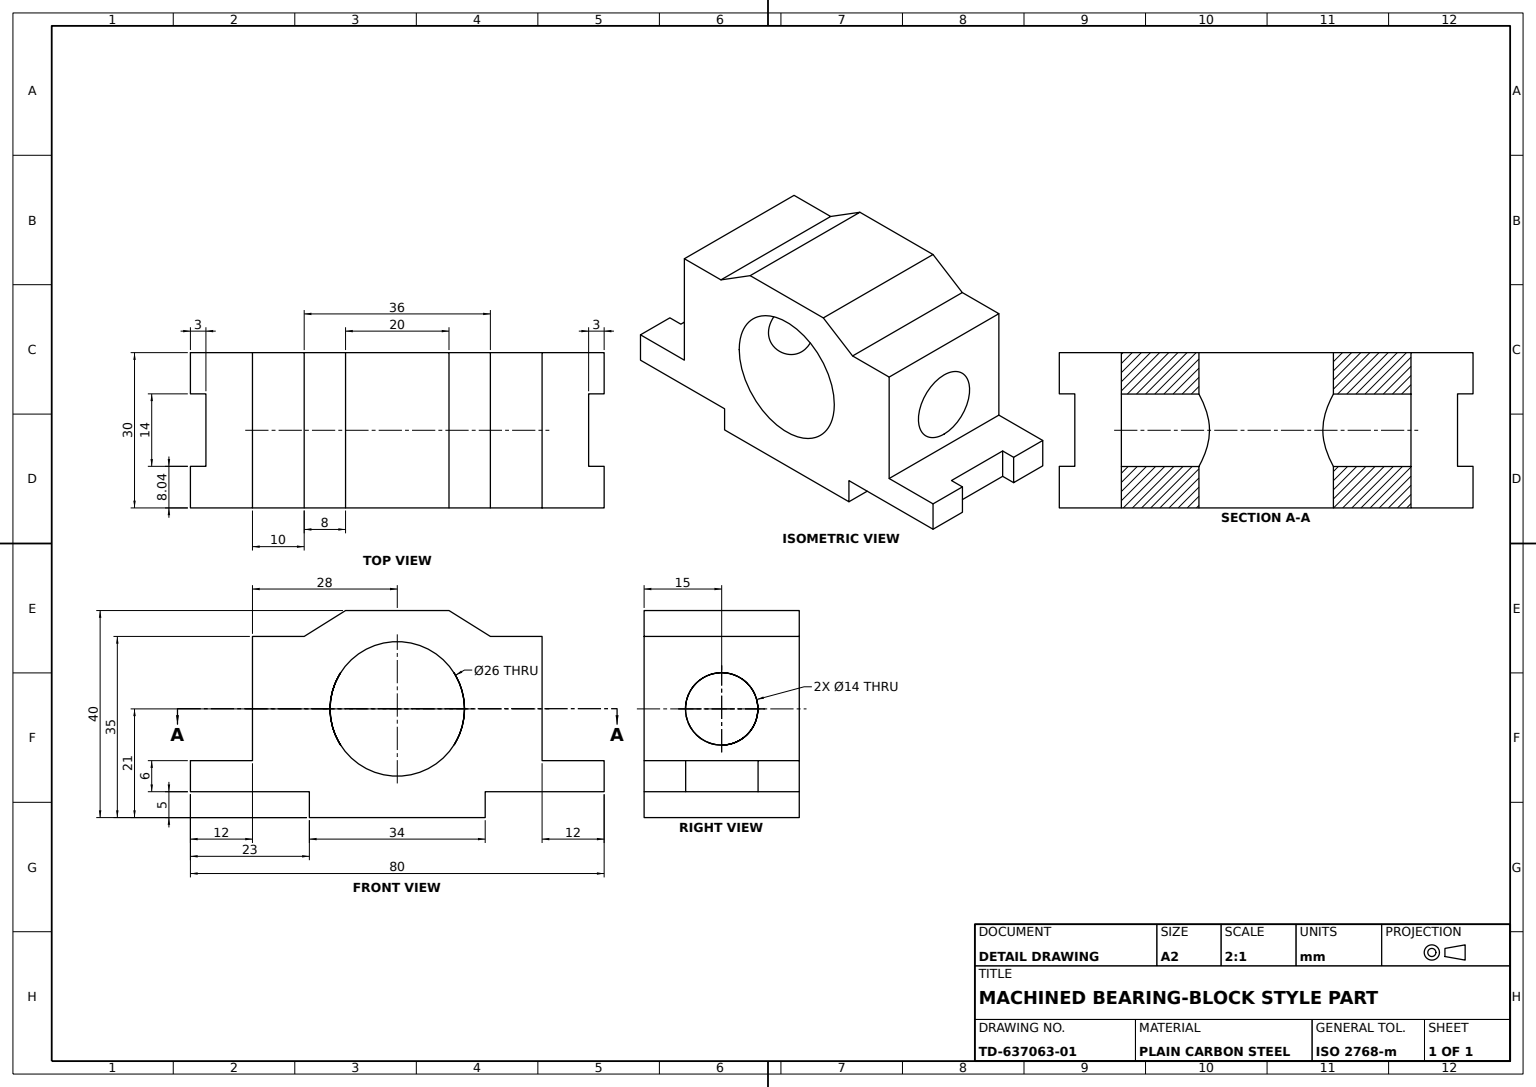
from build123d import *

# Parameters (mm, degrees)
BLOCK_PROFILE_SKETCH_R   = 13
BLOCK_BODY_DEPTH         = 30
TOP_GROOVE_SKETCH_W      = 3
TOP_GROOVE_SKETCH_H      = 14
TOP_GROOVE_CUT_DEPTH     = 91.227490268
SIDE_CROSS_HOLE_SKETCH_R = 7
SIDE_CROSS_HOLE_DEPTH    = 83.152297594


with BuildPart() as part:
    # Block Profile Sketch → Block Body (new body)
    with BuildSketch(Plane.XY):
        Polygon((0, 0), (23, 0), (23, -5), (57, -5), (57, 0), (80, 0), (80, 6), (68, 6), (68, 30), (58, 30), (50, 35), (30, 35), (22, 30), (12, 30), (12, 6), (0, 6), align=None)
        with Locations((40, 16)):
            Circle(BLOCK_PROFILE_SKETCH_R, mode=Mode.SUBTRACT)
    extrude(amount=-BLOCK_BODY_DEPTH)

    # Top Groove Sketch → Top Groove Cut (cut, through all)
    with BuildSketch(Plane(origin=(0, 6, 0), x_dir=(1, 0, 0), z_dir=(0, 1, 0))):
        with Locations((1.5, 15.037121503)):
            Rectangle(TOP_GROOVE_SKETCH_W, TOP_GROOVE_SKETCH_H)
        with Locations((78.5, 15.037121503)):
            Rectangle(TOP_GROOVE_SKETCH_W, TOP_GROOVE_SKETCH_H)
    extrude(amount=-TOP_GROOVE_CUT_DEPTH, mode=Mode.SUBTRACT)

    # Side Cross Hole Sketch → Side Cross Hole (cut, through all)
    with BuildSketch(Plane.ZY.offset(-12)):
        with Locations(Location((-15, 16, 0), (0, 0, 270))):
            Circle(SIDE_CROSS_HOLE_SKETCH_R)
    extrude(amount=-SIDE_CROSS_HOLE_DEPTH, mode=Mode.SUBTRACT)


solid = part.part
